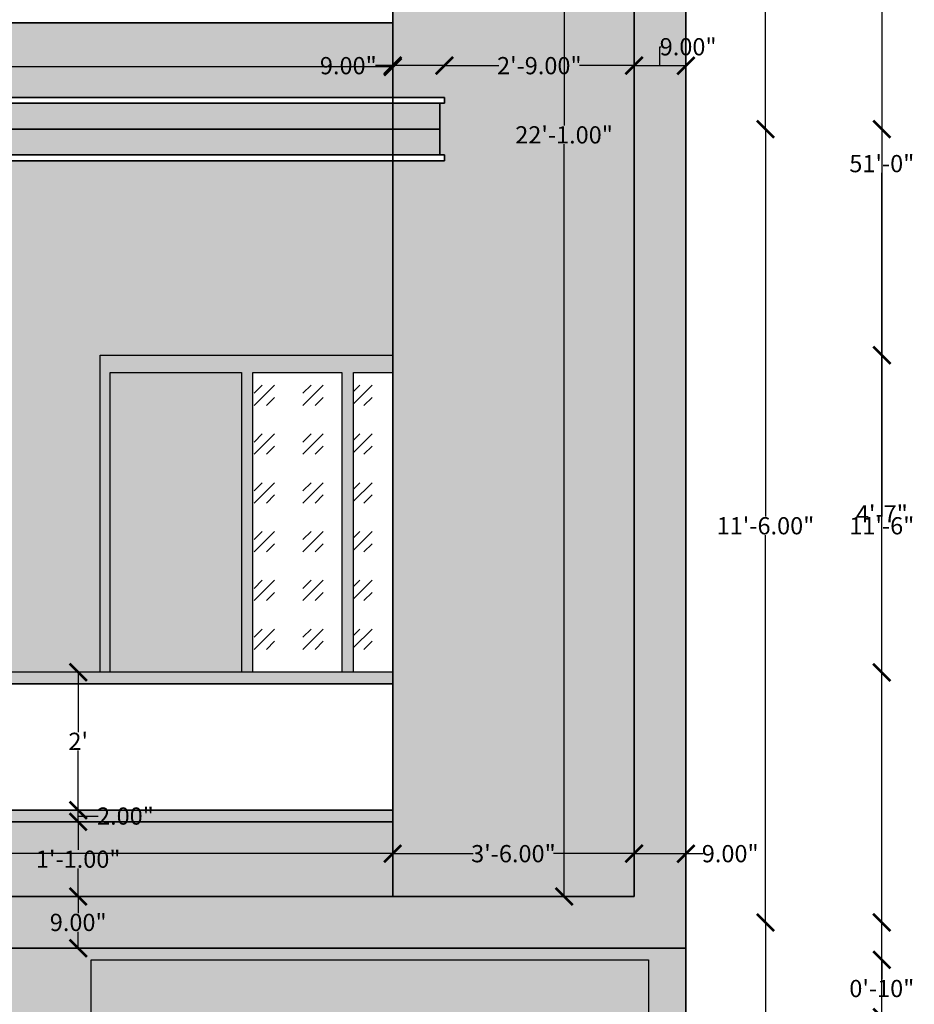
# Model space of a CAD drawing. Units: inches. Extents: x -654 to 390, y -40 to 648.
# Tile 8 of 13: x 231 to 386, y 159 to 330. Entities that reach past the tile are written whole.
import ezdxf

# ---------------------------------------------------------------- set-up
doc = ezdxf.new("R2010")
doc.units = ezdxf.units.IN
doc.header["$PDMODE"] = 3
for name, color, linetype, lineweight in [('A-ANNO-DIMS', 2, 'Continuous', 18), ('A-DOOR', 3, 'Continuous', 25), ('A-ELEV', 7, 'Continuous', 35), ('A-ELEV-FILL', 252, 'Continuous', 13), ('A-ELEV-PATT', 8, 'Continuous', 13), ('A-GLAZ', 4, 'Continuous', 25)]:
    doc.layers.add(name, color=color, linetype=linetype, lineweight=lineweight)
doc.styles.get("Standard").update_dxf_attribs({"font": 'arial.ttf'})
doc.dimstyles.get("Standard").update_dxf_attribs({"dimtxt": 3, "dimasz": 3, "dimexe": 0.18, "dimexo": 0.0625, "dimgap": 0.09, "dimtad": 0, "dimtih": 1, "dimtoh": 1, "dimzin": 0, "dimdsep": 46, "dimlunit": 3, "dimtxsty": 'Standard', "dimblk": 'ARCHTICK', "dimcen": 0.09, "dimse1": 1, "dimse2": 1, "dimadec": 0, "dimazin": 0, "dimtfac": 1, "dimtofl": 0, "dimtmove": 0, "dimatfit": 3, "dimfxl": 1, "dimtolj": 1, "dimtzin": 0, "dimarcsym": 0})

# ---------------------------------------------------------------- blocks, each defined once
blk = doc.blocks.new('_ArchTick')
at = {"color": 0, "linetype": 'ByBlock', "const_width": 0.15}
blk.add_lwpolyline([(-0.5, -0.5), (0.5, 0.5)], dxfattribs=at)
blk = doc.blocks.new('*D4')
at = {"layer": 'A-ANNO-DIMS', "color": 0, "lineweight": -2, "transparency": 16777216}
for p, q in [((360.51, 173.13), (360.51, 105.76)), ((360.51, 35.13), (360.51, 102.51))]:
    blk.add_line(p, q, dxfattribs=at)
at = {"layer": 'Defpoints', "color": 0, "transparency": 16777216}
for p in [(346.65, 173.13), (360.51, 173.13), (346.65, 35.13)]:
    blk.add_point(p, dxfattribs=at)
at = {"layer": 'A-ANNO-DIMS', "color": 0, "lineweight": -2, "transparency": 16777216, "xscale": 3, "yscale": 3, "zscale": 3}
for p, rotation in [((360.51, 173.13), 90), ((360.51, 35.13), 270)]:
    blk.add_blockref('_ArchTick', p, dxfattribs=dict(at, rotation=rotation))
at = {"layer": 'A-ANNO-DIMS', "color": 0, "transparency": 16777216, "insert": (360.51, 104.13), "char_height": 3, "attachment_point": 5}
blk.add_mtext('\\A1;11\'-6.00"', dxfattribs=at)
blk = doc.blocks.new('*D5')
at = {"layer": 'A-ANNO-DIMS', "color": 0, "lineweight": -2, "transparency": 16777216}
for p, q in [((360.51, 311.13), (360.51, 243.76)), ((360.51, 173.13), (360.51, 240.51))]:
    blk.add_line(p, q, dxfattribs=at)
at = {"layer": 'Defpoints', "color": 0, "transparency": 16777216}
for p in [(303.82, 311.13), (360.51, 311.13), (346.65, 173.13)]:
    blk.add_point(p, dxfattribs=at)
at = {"layer": 'A-ANNO-DIMS', "color": 0, "lineweight": -2, "transparency": 16777216, "xscale": 3, "yscale": 3, "zscale": 3}
for p, rotation in [((360.51, 311.13), 90), ((360.51, 173.13), 270)]:
    blk.add_blockref('_ArchTick', p, dxfattribs=dict(at, rotation=rotation))
at = {"layer": 'A-ANNO-DIMS', "color": 0, "transparency": 16777216, "insert": (360.51, 242.13), "char_height": 3, "attachment_point": 5}
blk.add_mtext('\\A1;11\'-6.00"', dxfattribs=at)
blk = doc.blocks.new('*D6')
at = {"layer": 'A-ANNO-DIMS', "color": 0, "lineweight": -2, "transparency": 16777216}
for p, q in [((360.51, 449.13), (360.51, 381.76)), ((360.51, 311.13), (360.51, 378.51))]:
    blk.add_line(p, q, dxfattribs=at)
at = {"layer": 'Defpoints', "color": 0, "transparency": 16777216}
for p in [(337.55, 449.13), (360.51, 449.13), (303.82, 311.13)]:
    blk.add_point(p, dxfattribs=at)
at = {"layer": 'A-ANNO-DIMS', "color": 0, "lineweight": -2, "transparency": 16777216, "xscale": 3, "yscale": 3, "zscale": 3}
for p, rotation in [((360.51, 449.13), 90), ((360.51, 311.13), 270)]:
    blk.add_blockref('_ArchTick', p, dxfattribs=dict(at, rotation=rotation))
at = {"layer": 'A-ANNO-DIMS', "color": 0, "transparency": 16777216, "insert": (360.51, 380.13), "char_height": 3, "attachment_point": 5}
blk.add_mtext('\\A1;11\'-6.00"', dxfattribs=at)
blk = doc.blocks.new('*D41')
at = {"layer": 'A-ANNO-DIMS', "color": 0, "lineweight": -2, "transparency": 16777216}
for p, q in [((325.46, 442.63), (325.46, 311.76)), ((325.46, 177.63), (325.46, 308.51))]:
    blk.add_line(p, q, dxfattribs=at)
at = {"layer": 'Defpoints', "color": 0, "transparency": 16777216}
for p in [(295.65, 442.63), (295.65, 177.63), (325.46, 177.63)]:
    blk.add_point(p, dxfattribs=at)
at = {"layer": 'A-ANNO-DIMS', "color": 0, "lineweight": -2, "transparency": 16777216, "xscale": 3, "yscale": 3, "zscale": 3}
for p, rotation in [((325.46, 442.63), 90), ((325.46, 177.63), 270)]:
    blk.add_blockref('_ArchTick', p, dxfattribs=dict(at, rotation=rotation))
at = {"layer": 'A-ANNO-DIMS', "color": 0, "transparency": 16777216, "insert": (325.46, 310.13), "char_height": 3, "attachment_point": 5}
blk.add_mtext('\\A1;22\'-1.00"', dxfattribs=at)
blk = doc.blocks.new('*D42')
at = {"layer": 'A-ANNO-DIMS', "color": 0, "lineweight": -2, "transparency": 16777216}
for p, q in [((304.65, 322.17), (314.13, 322.17)), ((337.65, 322.17), (328.16, 322.17))]:
    blk.add_line(p, q, dxfattribs=at)
at = {"layer": 'Defpoints', "color": 0, "transparency": 16777216}
for p in [(337.65, 322.17), (304.65, 316.63), (337.65, 316.63)]:
    blk.add_point(p, dxfattribs=at)
at = {"layer": 'A-ANNO-DIMS', "color": 0, "lineweight": -2, "transparency": 16777216, "xscale": 3, "yscale": 3, "zscale": 3, "rotation": 180}
blk.add_blockref('_ArchTick', (304.65, 322.17), dxfattribs=at)
at = {"layer": 'A-ANNO-DIMS', "color": 0, "lineweight": -2, "transparency": 16777216, "xscale": 3, "yscale": 3, "zscale": 3}
blk.add_blockref('_ArchTick', (337.65, 322.17), dxfattribs=at)
at = {"layer": 'A-ANNO-DIMS', "color": 0, "transparency": 16777216, "insert": (321.15, 322.17), "char_height": 3, "attachment_point": 5}
blk.add_mtext('\\A1;2\'-9.00"', dxfattribs=at)
blk = doc.blocks.new('*D43')
at = {"layer": 'A-ANNO-DIMS', "color": 0, "lineweight": -2, "transparency": 16777216}
for p, q in [((342.15, 322.17), (342.15, 325.46)), ((342.15, 325.46), (342.33, 325.46)), ((337.65, 322.17), (346.65, 322.17))]:
    blk.add_line(p, q, dxfattribs=at)
at = {"layer": 'Defpoints', "color": 0, "transparency": 16777216}
for p in [(346.65, 322.17), (346.65, 322.17), (337.65, 316.63)]:
    blk.add_point(p, dxfattribs=at)
at = {"layer": 'A-ANNO-DIMS', "color": 0, "lineweight": -2, "transparency": 16777216, "xscale": 3, "yscale": 3, "zscale": 3, "rotation": 180}
blk.add_blockref('_ArchTick', (337.65, 322.17), dxfattribs=at)
at = {"layer": 'A-ANNO-DIMS', "color": 0, "lineweight": -2, "transparency": 16777216, "xscale": 3, "yscale": 3, "zscale": 3}
blk.add_blockref('_ArchTick', (346.65, 322.17), dxfattribs=at)
at = {"layer": 'A-ANNO-DIMS', "color": 0, "transparency": 16777216, "insert": (347.05, 325.46), "char_height": 3, "attachment_point": 5}
blk.add_mtext('\\A1;9.00"', dxfattribs=at)
blk = doc.blocks.new('*D44')
at = {"layer": 'A-ANNO-DIMS', "color": 0, "lineweight": -2, "transparency": 16777216}
for p, q in [((295.65, 322.17), (292.65, 322.17)), ((304.65, 322.17), (295.65, 322.17))]:
    blk.add_line(p, q, dxfattribs=at)
at = {"layer": 'Defpoints', "color": 0, "transparency": 16777216}
for p in [(295.65, 322.17), (295.65, 316.63), (304.65, 316.63)]:
    blk.add_point(p, dxfattribs=at)
at = {"layer": 'A-ANNO-DIMS', "color": 0, "lineweight": -2, "transparency": 16777216, "xscale": 3, "yscale": 3, "zscale": 3, "rotation": 180}
blk.add_blockref('_ArchTick', (295.65, 322.17), dxfattribs=at)
at = {"layer": 'A-ANNO-DIMS', "color": 0, "lineweight": -2, "transparency": 16777216, "xscale": 3, "yscale": 3, "zscale": 3}
blk.add_blockref('_ArchTick', (304.65, 322.17), dxfattribs=at)
at = {"layer": 'A-ANNO-DIMS', "color": 0, "transparency": 16777216, "insert": (287.92, 322.17), "char_height": 3, "attachment_point": 5}
blk.add_mtext('\\A1;9.00"', dxfattribs=at)
blk = doc.blocks.new('*D46')
at = {"layer": 'A-ANNO-DIMS', "color": 0, "lineweight": -2, "transparency": 16777216}
for p, q in [((145.65, 321.96), (212.63, 321.96)), ((295.65, 321.96), (228.66, 321.96))]:
    blk.add_line(p, q, dxfattribs=at)
at = {"layer": 'Defpoints', "color": 0, "transparency": 16777216}
for p in [(145.65, 329.63), (145.65, 321.96), (295.65, 316.63)]:
    blk.add_point(p, dxfattribs=at)
at = {"layer": 'A-ANNO-DIMS', "color": 0, "lineweight": -2, "transparency": 16777216, "xscale": 3, "yscale": 3, "zscale": 3, "rotation": 180}
blk.add_blockref('_ArchTick', (145.65, 321.96), dxfattribs=at)
at = {"layer": 'A-ANNO-DIMS', "color": 0, "lineweight": -2, "transparency": 16777216, "xscale": 3, "yscale": 3, "zscale": 3}
blk.add_blockref('_ArchTick', (295.65, 321.96), dxfattribs=at)
at = {"layer": 'A-ANNO-DIMS', "color": 0, "transparency": 16777216, "insert": (220.65, 321.96), "char_height": 3, "attachment_point": 5}
blk.add_mtext('\\A1;12\'-6.00"', dxfattribs=at)
blk = doc.blocks.new('*D58')
at = {"layer": 'A-ANNO-DIMS', "color": 0, "lineweight": -2, "transparency": 16777216}
for p, q in [((337.65, 185.09), (346.65, 185.09)), ((346.65, 185.09), (349.65, 185.09))]:
    blk.add_line(p, q, dxfattribs=at)
at = {"layer": 'Defpoints', "color": 0, "transparency": 16777216}
for p in [(346.65, 185.09), (337.65, 177.63), (346.65, 177.63)]:
    blk.add_point(p, dxfattribs=at)
at = {"layer": 'A-ANNO-DIMS', "color": 0, "lineweight": -2, "transparency": 16777216, "xscale": 3, "yscale": 3, "zscale": 3, "rotation": 180}
blk.add_blockref('_ArchTick', (337.65, 185.09), dxfattribs=at)
at = {"layer": 'A-ANNO-DIMS', "color": 0, "lineweight": -2, "transparency": 16777216, "xscale": 3, "yscale": 3, "zscale": 3}
blk.add_blockref('_ArchTick', (346.65, 185.09), dxfattribs=at)
at = {"layer": 'A-ANNO-DIMS', "color": 0, "transparency": 16777216, "insert": (354.37, 185.09), "char_height": 3, "attachment_point": 5}
blk.add_mtext('\\A1;9.00"', dxfattribs=at)
blk = doc.blocks.new('*D59')
at = {"layer": 'A-ANNO-DIMS', "color": 0, "lineweight": -2, "transparency": 16777216}
for p, q in [((295.65, 185.09), (309.66, 185.09)), ((337.65, 185.09), (323.64, 185.09))]:
    blk.add_line(p, q, dxfattribs=at)
at = {"layer": 'Defpoints', "color": 0, "transparency": 16777216}
for p in [(295.65, 185.09), (295.65, 185.09), (337.65, 185.09)]:
    blk.add_point(p, dxfattribs=at)
at = {"layer": 'A-ANNO-DIMS', "color": 0, "lineweight": -2, "transparency": 16777216, "xscale": 3, "yscale": 3, "zscale": 3, "rotation": 180}
blk.add_blockref('_ArchTick', (295.65, 185.09), dxfattribs=at)
at = {"layer": 'A-ANNO-DIMS', "color": 0, "lineweight": -2, "transparency": 16777216, "xscale": 3, "yscale": 3, "zscale": 3}
blk.add_blockref('_ArchTick', (337.65, 185.09), dxfattribs=at)
at = {"layer": 'A-ANNO-DIMS', "color": 0, "transparency": 16777216, "insert": (316.65, 185.09), "char_height": 3, "attachment_point": 5}
blk.add_mtext('\\A1;3\'-6.00"', dxfattribs=at)
blk = doc.blocks.new('*D60')
at = {"layer": 'A-ANNO-DIMS', "color": 0, "lineweight": -2, "transparency": 16777216}
for p, q in [((120.15, 185.09), (199.88, 185.09)), ((295.65, 185.09), (215.91, 185.09))]:
    blk.add_line(p, q, dxfattribs=at)
at = {"layer": 'Defpoints', "color": 0, "transparency": 16777216}
for p in [(120.15, 185.09), (120.15, 185.09), (295.65, 185.09)]:
    blk.add_point(p, dxfattribs=at)
at = {"layer": 'A-ANNO-DIMS', "color": 0, "lineweight": -2, "transparency": 16777216, "xscale": 3, "yscale": 3, "zscale": 3, "rotation": 180}
blk.add_blockref('_ArchTick', (120.15, 185.09), dxfattribs=at)
at = {"layer": 'A-ANNO-DIMS', "color": 0, "lineweight": -2, "transparency": 16777216, "xscale": 3, "yscale": 3, "zscale": 3}
blk.add_blockref('_ArchTick', (295.65, 185.09), dxfattribs=at)
at = {"layer": 'A-ANNO-DIMS', "color": 0, "transparency": 16777216, "insert": (207.9, 185.09), "char_height": 3, "attachment_point": 5}
blk.add_mtext('\\A1;14\'-7.50"', dxfattribs=at)
blk = doc.blocks.new('*D62')
at = {"layer": 'A-ANNO-DIMS', "color": 0, "lineweight": -2, "transparency": 16777216}
for p, q in [((240.92, 190.63), (240.92, 185.76)), ((240.92, 177.63), (240.92, 182.51))]:
    blk.add_line(p, q, dxfattribs=at)
at = {"layer": 'Defpoints', "color": 0, "transparency": 16777216}
for p in [(240.92, 190.63), (295.65, 190.63), (295.65, 177.63)]:
    blk.add_point(p, dxfattribs=at)
at = {"layer": 'A-ANNO-DIMS', "color": 0, "lineweight": -2, "transparency": 16777216, "xscale": 3, "yscale": 3, "zscale": 3}
for p, rotation in [((240.92, 190.63), 90), ((240.92, 177.63), 270)]:
    blk.add_blockref('_ArchTick', p, dxfattribs=dict(at, rotation=rotation))
at = {"layer": 'A-ANNO-DIMS', "color": 0, "transparency": 16777216, "insert": (240.92, 184.13), "char_height": 3, "attachment_point": 5}
blk.add_mtext('\\A1;1\'-1.00"', dxfattribs=at)
blk = doc.blocks.new('*D63')
at = {"layer": 'A-ANNO-DIMS', "color": 0, "lineweight": -2, "transparency": 16777216}
for p, q in [((240.92, 190.63), (240.92, 192.63)), ((240.92, 191.63), (244.21, 191.63)), ((244.21, 191.63), (244.39, 191.63))]:
    blk.add_line(p, q, dxfattribs=at)
at = {"layer": 'Defpoints', "color": 0, "transparency": 16777216}
for p in [(240.92, 192.63), (240.92, 192.63), (295.65, 190.63)]:
    blk.add_point(p, dxfattribs=at)
at = {"layer": 'A-ANNO-DIMS', "color": 0, "lineweight": -2, "transparency": 16777216, "xscale": 3, "yscale": 3, "zscale": 3}
for p, rotation in [((240.92, 192.63), 90), ((240.92, 190.63), 270)]:
    blk.add_blockref('_ArchTick', p, dxfattribs=dict(at, rotation=rotation))
at = {"layer": 'A-ANNO-DIMS', "color": 0, "transparency": 16777216, "insert": (249.14, 191.63), "char_height": 3, "attachment_point": 5}
blk.add_mtext('\\A1;2.00"', dxfattribs=at)
blk = doc.blocks.new('*D64')
at = {"layer": 'A-ANNO-DIMS', "color": 0, "lineweight": -2, "transparency": 16777216}
for p, q in [((240.92, 216.63), (240.92, 206.23)), ((240.92, 192.63), (240.92, 203.04))]:
    blk.add_line(p, q, dxfattribs=at)
at = {"layer": 'Defpoints', "color": 0, "transparency": 16777216}
for p in [(240.92, 216.63), (240.92, 216.63), (240.92, 192.63)]:
    blk.add_point(p, dxfattribs=at)
at = {"layer": 'A-ANNO-DIMS', "color": 0, "lineweight": -2, "transparency": 16777216, "xscale": 3, "yscale": 3, "zscale": 3}
for p, rotation in [((240.92, 216.63), 90), ((240.92, 192.63), 270)]:
    blk.add_blockref('_ArchTick', p, dxfattribs=dict(at, rotation=rotation))
at = {"layer": 'A-ANNO-DIMS', "color": 0, "transparency": 16777216, "insert": (240.92, 204.63), "char_height": 3, "attachment_point": 5}
blk.add_mtext("\\A1;2'", dxfattribs=at)
blk = doc.blocks.new('*D71')
at = {"layer": 'A-ANNO-DIMS', "color": 0, "lineweight": -2, "transparency": 16777216}
for p, q in [((240.92, 177.63), (240.92, 174.76)), ((240.92, 168.63), (240.92, 171.51))]:
    blk.add_line(p, q, dxfattribs=at)
at = {"layer": 'Defpoints', "color": 0, "transparency": 16777216}
for p in [(240.92, 177.63), (240.92, 168.63), (240.92, 168.63)]:
    blk.add_point(p, dxfattribs=at)
at = {"layer": 'A-ANNO-DIMS', "color": 0, "lineweight": -2, "transparency": 16777216, "xscale": 3, "yscale": 3, "zscale": 3}
for p, rotation in [((240.92, 177.63), 90), ((240.92, 168.63), 270)]:
    blk.add_blockref('_ArchTick', p, dxfattribs=dict(at, rotation=rotation))
at = {"layer": 'A-ANNO-DIMS', "color": 0, "transparency": 16777216, "insert": (240.92, 173.13), "char_height": 3, "attachment_point": 5}
blk.add_mtext('\\A1;9.00"', dxfattribs=at)
blk = doc.blocks.new('*D76')
at = {"layer": 'A-ANNO-DIMS', "color": 0, "lineweight": -2, "transparency": 16777216}
for p, q in [((380.75, 611.13), (380.75, 306.76)), ((380.75, -0.87), (380.75, 303.51))]:
    blk.add_line(p, q, dxfattribs=at)
at = {"layer": 'Defpoints', "color": 0, "transparency": 16777216}
for p in [(126.65, 611.13), (380.75, 611.13), (346.65, -0.87)]:
    blk.add_point(p, dxfattribs=at)
at = {"layer": 'A-ANNO-DIMS', "color": 0, "lineweight": -2, "transparency": 16777216, "xscale": 3, "yscale": 3, "zscale": 3}
for p, rotation in [((380.75, 611.13), 90), ((380.75, -0.87), 270)]:
    blk.add_blockref('_ArchTick', p, dxfattribs=dict(at, rotation=rotation))
at = {"layer": 'A-ANNO-DIMS', "color": 0, "transparency": 16777216, "insert": (380.75, 305.13), "char_height": 3, "attachment_point": 5}
blk.add_mtext('\\A1;51\'-0"', dxfattribs=at)
blk = doc.blocks.new('*D89')
at = {"layer": 'A-ANNO-DIMS', "color": 0, "lineweight": -2, "transparency": 16777216}
for p, q in [((243.65, 643.23), (287.57, 643.23)), ((339.65, 643.23), (295.73, 643.23))]:
    blk.add_line(p, q, dxfattribs=at)
at = {"layer": 'Defpoints', "color": 0, "transparency": 16777216}
for p in [(339.65, 643.23), (243.65, 17.13), (339.65, 17.13)]:
    blk.add_point(p, dxfattribs=at)
at = {"layer": 'A-ANNO-DIMS', "color": 0, "lineweight": -2, "transparency": 16777216, "xscale": 3, "yscale": 3, "zscale": 3, "rotation": 180}
blk.add_blockref('_ArchTick', (243.65, 643.23), dxfattribs=at)
at = {"layer": 'A-ANNO-DIMS', "color": 0, "lineweight": -2, "transparency": 16777216, "xscale": 3, "yscale": 3, "zscale": 3}
blk.add_blockref('_ArchTick', (339.65, 643.23), dxfattribs=at)
at = {"layer": 'A-ANNO-DIMS', "color": 0, "transparency": 16777216, "insert": (291.65, 643.23), "char_height": 3, "attachment_point": 5}
blk.add_mtext('\\A1;8\'-0"', dxfattribs=at)
blk = doc.blocks.new('*D90')
at = {"layer": 'A-ANNO-DIMS', "color": 0, "lineweight": -2, "transparency": 16777216}
for p, q in [((339.65, 643.23), (346.65, 643.23)), ((346.65, 643.23), (349.65, 643.23))]:
    blk.add_line(p, q, dxfattribs=at)
at = {"layer": 'Defpoints', "color": 0, "transparency": 16777216}
for p in [(346.65, 643.23), (339.65, 17.13), (346.65, 17.13)]:
    blk.add_point(p, dxfattribs=at)
at = {"layer": 'A-ANNO-DIMS', "color": 0, "lineweight": -2, "transparency": 16777216, "xscale": 3, "yscale": 3, "zscale": 3, "rotation": 180}
blk.add_blockref('_ArchTick', (339.65, 643.23), dxfattribs=at)
at = {"layer": 'A-ANNO-DIMS', "color": 0, "lineweight": -2, "transparency": 16777216, "xscale": 3, "yscale": 3, "zscale": 3}
blk.add_blockref('_ArchTick', (346.65, 643.23), dxfattribs=at)
at = {"layer": 'A-ANNO-DIMS', "color": 0, "transparency": 16777216, "insert": (353.72, 643.23), "char_height": 3, "attachment_point": 5}
blk.add_mtext('\\A1;0\'-7"', dxfattribs=at)
blk = doc.blocks.new('*D91')
at = {"layer": 'A-ANNO-DIMS', "color": 0, "lineweight": -2, "transparency": 16777216}
for p, q in [((380.75, 166.63), (380.75, 163.26)), ((380.75, 156.63), (380.75, 160.01))]:
    blk.add_line(p, q, dxfattribs=at)
at = {"layer": 'Defpoints', "color": 0, "transparency": 16777216}
for p in [(243.15, 166.63), (380.75, 166.63), (243.15, 156.63)]:
    blk.add_point(p, dxfattribs=at)
at = {"layer": 'A-ANNO-DIMS', "color": 0, "lineweight": -2, "transparency": 16777216, "xscale": 3, "yscale": 3, "zscale": 3}
for p, rotation in [((380.75, 166.63), 90), ((380.75, 156.63), 270)]:
    blk.add_blockref('_ArchTick', p, dxfattribs=dict(at, rotation=rotation))
at = {"layer": 'A-ANNO-DIMS', "color": 0, "transparency": 16777216, "insert": (380.75, 161.63), "char_height": 3, "attachment_point": 5}
blk.add_mtext('\\A1;0\'-10"', dxfattribs=at)
blk = doc.blocks.new('*D94')
at = {"layer": 'A-ANNO-DIMS', "color": 0, "lineweight": -2, "transparency": 16777216}
for p, q in [((380.75, 271.79), (380.75, 245.8)), ((380.75, 216.63), (380.75, 242.62))]:
    blk.add_line(p, q, dxfattribs=at)
at = {"layer": 'Defpoints', "color": 0, "transparency": 16777216}
for p in [(221.33, 271.79), (244.73, 216.63), (380.75, 216.63)]:
    blk.add_point(p, dxfattribs=at)
at = {"layer": 'A-ANNO-DIMS', "color": 0, "lineweight": -2, "transparency": 16777216, "xscale": 3, "yscale": 3, "zscale": 3}
for p, rotation in [((380.75, 271.79), 90), ((380.75, 216.63), 270)]:
    blk.add_blockref('_ArchTick', p, dxfattribs=dict(at, rotation=rotation))
at = {"layer": 'A-ANNO-DIMS', "color": 0, "transparency": 16777216, "insert": (380.75, 244.21), "char_height": 3, "attachment_point": 5}
blk.add_mtext('\\A1;4\'-7"', dxfattribs=at)
blk = doc.blocks.new('*D95')
at = {"layer": 'A-ANNO-DIMS', "color": 0, "lineweight": -2, "transparency": 16777216}
for p, q in [((244.73, -32.97), (266.05, -32.97)), ((295.65, -32.97), (274.32, -32.97))]:
    blk.add_line(p, q, dxfattribs=at)
at = {"layer": 'Defpoints', "color": 0, "transparency": 16777216}
for p in [(244.73, 271.79), (295.65, 271.79), (295.65, -32.97)]:
    blk.add_point(p, dxfattribs=at)
at = {"layer": 'A-ANNO-DIMS', "color": 0, "lineweight": -2, "transparency": 16777216, "xscale": 3, "yscale": 3, "zscale": 3, "rotation": 180}
blk.add_blockref('_ArchTick', (244.73, -32.97), dxfattribs=at)
at = {"layer": 'A-ANNO-DIMS', "color": 0, "lineweight": -2, "transparency": 16777216, "xscale": 3, "yscale": 3, "zscale": 3}
blk.add_blockref('_ArchTick', (295.65, -32.97), dxfattribs=at)
at = {"layer": 'A-ANNO-DIMS', "color": 0, "transparency": 16777216, "insert": (270.19, -32.97), "char_height": 3, "attachment_point": 5}
blk.add_mtext('\\A1;4\'-3"', dxfattribs=at)
blk = doc.blocks.new('*D99')
at = {"layer": 'A-ANNO-DIMS', "color": 0, "lineweight": -2, "transparency": 16777216}
for p, q in [((380.75, 311.13), (380.75, 243.76)), ((380.75, 173.13), (380.75, 240.51))]:
    blk.add_line(p, q, dxfattribs=at)
at = {"layer": 'Defpoints', "color": 0, "transparency": 16777216}
for p in [(178.74, 311.13), (380.75, 311.13), (178.74, 173.13)]:
    blk.add_point(p, dxfattribs=at)
at = {"layer": 'A-ANNO-DIMS', "color": 0, "lineweight": -2, "transparency": 16777216, "xscale": 3, "yscale": 3, "zscale": 3}
for p, rotation in [((380.75, 311.13), 90), ((380.75, 173.13), 270)]:
    blk.add_blockref('_ArchTick', p, dxfattribs=dict(at, rotation=rotation))
at = {"layer": 'A-ANNO-DIMS', "color": 0, "transparency": 16777216, "insert": (380.75, 242.13), "char_height": 3, "attachment_point": 5}
blk.add_mtext('\\A1;11\'-6"', dxfattribs=at)
blk = doc.blocks.new('*D102')
at = {"layer": 'A-ANNO-DIMS', "color": 0, "lineweight": -2, "transparency": 16777216}
for p, q in [((179.88, -32.97), (205.8, -32.97)), ((239.87, -32.97), (213.95, -32.97))]:
    blk.add_line(p, q, dxfattribs=at)
at = {"layer": 'Defpoints', "color": 0, "transparency": 16777216}
for p in [(179.88, 355.63), (239.87, 355.63), (239.87, -32.97)]:
    blk.add_point(p, dxfattribs=at)
at = {"layer": 'A-ANNO-DIMS', "color": 0, "lineweight": -2, "transparency": 16777216, "xscale": 3, "yscale": 3, "zscale": 3, "rotation": 180}
blk.add_blockref('_ArchTick', (179.88, -32.97), dxfattribs=at)
at = {"layer": 'A-ANNO-DIMS', "color": 0, "lineweight": -2, "transparency": 16777216, "xscale": 3, "yscale": 3, "zscale": 3}
blk.add_blockref('_ArchTick', (239.87, -32.97), dxfattribs=at)
at = {"layer": 'A-ANNO-DIMS', "color": 0, "transparency": 16777216, "insert": (209.87, -32.97), "char_height": 3, "attachment_point": 5}
blk.add_mtext('\\A1;5\'-0"', dxfattribs=at)
blk = doc.blocks.new('*D103')
at = {"layer": 'A-ANNO-DIMS', "color": 0, "lineweight": -2, "transparency": 16777216}
for p, q in [((239.87, -32.97), (257.87, -32.97)), ((291.14, -32.97), (273.14, -32.97))]:
    blk.add_line(p, q, dxfattribs=at)
at = {"layer": 'Defpoints', "color": 0, "transparency": 16777216}
for p in [(239.87, 355.63), (291.14, 355.63), (291.14, -32.97)]:
    blk.add_point(p, dxfattribs=at)
at = {"layer": 'A-ANNO-DIMS', "color": 0, "lineweight": -2, "transparency": 16777216, "xscale": 3, "yscale": 3, "zscale": 3, "rotation": 180}
blk.add_blockref('_ArchTick', (239.87, -32.97), dxfattribs=at)
at = {"layer": 'A-ANNO-DIMS', "color": 0, "lineweight": -2, "transparency": 16777216, "xscale": 3, "yscale": 3, "zscale": 3}
blk.add_blockref('_ArchTick', (291.14, -32.97), dxfattribs=at)
at = {"layer": 'A-ANNO-DIMS', "color": 0, "transparency": 16777216, "insert": (265.51, -32.97), "char_height": 3, "attachment_point": 5}
blk.add_mtext('\\A1;4\'-3 1/2"', dxfattribs=at)

msp = doc.modelspace()

# ---------------------------------------------------------------- hatches: boundary and pattern name
at = {"layer": 'A-ELEV-FILL'}
h = msp.add_hatch(color=256, dxfattribs=at)
h.dxf.hatch_style = 1
h.paths.add_polyline_path([(161.035, 590.134), (-1.354, 590.134), (-1.354, 581.134), (161.035, 581.134)])
h.paths.add_polyline_path([(346.646, 453.634), (-1.354, 453.634), (-1.354, 444.634), (337.646, 444.634), (337.646, 177.634), (178.742, 177.634), (178.742, 173.134), (176.742, 173.134), (176.742, 177.634), (166.742, 177.634), (166.742, 173.134), (164.742, 173.134), (164.742, 177.634), (154.742, 177.634), (154.742, 173.134), (152.742, 173.134), (152.742, 177.634), (142.742, 177.634), (142.742, 173.134), (140.742, 173.134), (140.742, 177.634), (130.742, 177.634), (130.742, 173.134), (128.742, 173.134), (128.742, 177.634), (115.646, 177.634), (115.646, 168.634), (346.646, 168.634), (346.646, 173.134)])
h.paths.add_polyline_path([(7.646, 87.642), (-1.354, 87.642), (-1.354, 17.134), (7.646, 17.134)])
h.paths.add_polyline_path([(16.396, 116.134), (60.646, 116.134), (60.646, 83.134), (62.646, 83.134), (113.646, 83.134), (115.646, 83.134), (115.646, 125.134), (7.646, 125.134), (7.646, 89.642), (8.146, 89.642), (8.146, 87.642), (7.646, 87.642), (7.646, 83.134), (9.646, 83.134), (16.396, 83.134)])
h = msp.add_hatch(color=256, dxfattribs=at)
h.dxf.hatch_style = 1
h.paths.add_polyline_path([(346.646, 587.634), (161.035, 587.634), (161.035, 583.634), (342.646, 583.634), (342.646, 497.134), (346.646, 497.134), (346.646, 583.634)])
h.paths.add_polyline_path([(295.646, 315.634), (98.293, 315.634), (98.293, 311.134), (295.646, 311.134)])
h.paths.add_polyline_path([(128.742, 311.134), (98.293, 311.134), (98.293, 306.634), (128.742, 306.634)])
h.paths.add_polyline_path([(140.742, 311.134), (130.742, 311.134), (130.742, 306.634), (140.742, 306.634)])
h.paths.add_polyline_path([(152.742, 311.134), (142.742, 311.134), (142.742, 306.634), (152.742, 306.634)])
h.paths.add_polyline_path([(164.742, 311.134), (154.742, 311.134), (154.742, 306.634), (164.742, 306.634)])
h.paths.add_polyline_path([(176.742, 311.134), (166.742, 311.134), (166.742, 306.634), (176.742, 306.634)])
h.paths.add_polyline_path([(295.646, 311.134), (178.742, 311.134), (178.742, 306.634), (295.646, 306.634)])
h.paths.add_polyline_path([(303.818, 315.634), (295.646, 315.634), (295.646, 311.134), (303.818, 311.134)])
h.paths.add_polyline_path([(303.818, 311.134), (295.646, 311.134), (295.646, 306.634), (303.818, 306.634)])
h = msp.add_hatch(color=256, dxfattribs=at)
h.dxf.hatch_style = 1
h.paths.add_polyline_path([(41.55, 80.08), (28.05, 80.08), (28.05, 20.08), (41.55, 20.08)])
h.paths.add_polyline_path([(93.843, 80.08), (80.343, 80.08), (80.343, 20.08), (93.843, 20.08)])
h.paths.add_polyline_path([(337.646, 442.634), (295.646, 442.634), (295.646, 316.634), (304.646, 316.634), (304.646, 315.634), (303.818, 315.634), (303.818, 306.634), (304.646, 306.634), (304.646, 305.634), (295.646, 305.634), (295.646, 177.634), (337.646, 177.634)])
h.paths.add_polyline_path([(346.646, 495.134), (184.646, 495.134), (184.646, 453.634), (346.646, 453.634)])
h.paths.add_polyline_path([(198.646, 473.634), (198.646, 486.134), (332.646, 486.134), (332.646, 473.634)], flags=16)
h.paths.add_polyline_path([(199.646, 474.634), (199.646, 485.134), (331.646, 485.134), (331.646, 474.634)], flags=0)
h = msp.add_hatch(color=256, dxfattribs=at)
h.dxf.hatch_style = 1
h.paths.add_polyline_path([(295.646, 190.634), (178.742, 190.634), (178.742, 177.634), (295.646, 177.634)])
h.paths.add_polyline_path([(176.742, 190.634), (166.742, 190.634), (166.742, 177.634), (176.742, 177.634)])
h.paths.add_polyline_path([(164.742, 190.634), (154.742, 190.634), (154.742, 177.634), (164.742, 177.634)])
h.paths.add_polyline_path([(152.742, 190.634), (142.742, 190.634), (142.742, 177.634), (152.742, 177.634)])
h.paths.add_polyline_path([(140.742, 190.634), (130.742, 190.634), (130.742, 177.634), (140.742, 177.634)])
h.paths.add_polyline_path([(128.742, 190.634), (120.146, 190.634), (120.146, 177.634), (128.742, 177.634)])
h.paths.add_polyline_path([(295.646, 329.634), (145.646, 329.634), (145.646, 442.634), (100.646, 442.634), (100.646, 316.634), (295.646, 316.634)])
h.paths.add_polyline_path([(138.646, 359.634), (107.646, 359.634), (107.646, 438.634), (138.646, 438.634)], flags=16)
h.paths.add_polyline_path([(136.646, 361.634), (109.646, 361.634), (109.646, 436.634), (136.646, 436.634)], flags=0)
h.paths.add_polyline_path([(184.646, 466.634), (7.646, 466.634), (7.646, 453.634), (184.646, 453.634)])
h.paths.add_polyline_path([(184.646, 494.634), (7.646, 494.634), (7.646, 492.634), (184.646, 492.634)])
h.paths.add_polyline_path([(10.336, 492.634), (9.336, 492.634), (9.336, 468.634), (10.336, 468.634)])
h.paths.add_polyline_path([(17.352, 492.634), (16.352, 492.634), (16.352, 468.634), (17.352, 468.634)])
h.paths.add_polyline_path([(24.368, 492.634), (23.368, 492.634), (23.368, 468.634), (24.368, 468.634)])
h.paths.add_polyline_path([(31.384, 492.634), (30.384, 492.634), (30.384, 468.634), (31.384, 468.634)])
h.paths.add_polyline_path([(38.4, 492.634), (37.4, 492.634), (37.4, 468.634), (38.4, 468.634)])
h.paths.add_polyline_path([(45.416, 492.634), (44.416, 492.634), (44.416, 468.634), (45.416, 468.634)])
h.paths.add_polyline_path([(52.432, 492.634), (51.432, 492.634), (51.432, 468.634), (52.432, 468.634)])
h.paths.add_polyline_path([(59.448, 492.634), (58.448, 492.634), (58.448, 468.634), (59.448, 468.634)])
h.paths.add_polyline_path([(66.464, 492.634), (65.464, 492.634), (65.464, 468.634), (66.464, 468.634)])
h.paths.add_polyline_path([(73.48, 492.634), (72.48, 492.634), (72.48, 468.634), (73.48, 468.634)])
h.paths.add_polyline_path([(80.496, 492.634), (79.496, 492.634), (79.496, 468.634), (80.496, 468.634)])
h.paths.add_polyline_path([(87.512, 492.634), (86.512, 492.634), (86.512, 468.634), (87.512, 468.634)])
h.paths.add_polyline_path([(94.528, 492.634), (93.528, 492.634), (93.528, 468.634), (94.528, 468.634)])
h.paths.add_polyline_path([(101.544, 492.634), (100.544, 492.634), (100.544, 468.634), (101.544, 468.634)])
h.paths.add_polyline_path([(108.559, 492.634), (107.559, 492.634), (107.559, 468.634), (108.559, 468.634)])
h.paths.add_polyline_path([(115.575, 492.634), (114.575, 492.634), (114.575, 468.634), (115.575, 468.634)])
h.paths.add_polyline_path([(122.591, 492.634), (121.591, 492.634), (121.591, 468.634), (122.591, 468.634)])
h.paths.add_polyline_path([(129.607, 492.634), (128.607, 492.634), (128.607, 468.634), (129.607, 468.634)])
h.paths.add_polyline_path([(136.623, 492.634), (135.623, 492.634), (135.623, 468.634), (136.623, 468.634)])
h.paths.add_polyline_path([(143.639, 492.634), (142.639, 492.634), (142.639, 468.634), (143.639, 468.634)])
h.paths.add_polyline_path([(150.655, 492.634), (149.655, 492.634), (149.655, 468.634), (150.655, 468.634)])
h.paths.add_polyline_path([(157.671, 492.634), (156.671, 492.634), (156.671, 468.634), (157.671, 468.634)])
h.paths.add_polyline_path([(164.687, 492.634), (163.687, 492.634), (163.687, 468.634), (164.687, 468.634)])
h.paths.add_polyline_path([(171.703, 492.634), (170.703, 492.634), (170.703, 468.634), (171.703, 468.634)])
h.paths.add_polyline_path([(178.719, 492.634), (177.719, 492.634), (177.719, 468.634), (178.719, 468.634)])
h = msp.add_hatch(color=256, dxfattribs=at)
h.dxf.hatch_style = 1
h.paths.add_polyline_path([(138.646, 438.634), (107.646, 438.634), (107.646, 359.634), (138.646, 359.634)])
h.paths.add_polyline_path([(136.646, 436.634), (136.646, 361.634), (109.646, 361.634), (109.646, 436.634)], flags=16)
h.paths.add_polyline_path([(179.877, 410.786), (145.646, 410.786), (145.646, 407.786), (153.285, 407.786), (153.285, 357.634), (145.646, 357.634), (145.646, 355.634), (179.877, 355.634)])
h.paths.add_polyline_path([(178.123, 407.786), (178.123, 357.634), (155.286, 357.634), (155.286, 407.786)], flags=16)
h.paths.add_polyline_path([(291.141, 410.786), (239.871, 410.786), (239.871, 355.634), (241.996, 355.634), (241.996, 407.786), (269.317, 407.786), (269.317, 355.634), (271.318, 355.634), (271.318, 407.786), (289.369, 407.786), (289.369, 355.634), (291.141, 355.634)])
h.paths.add_polyline_path([(128.225, 268.786), (128.742, 268.786), (128.742, 271.786), (125.225, 271.786), (125.225, 216.634), (128.225, 216.634)])
h.paths.add_polyline_path([(140.742, 271.786), (130.742, 271.786), (130.742, 268.786), (140.742, 268.786)])
h.paths.add_polyline_path([(152.742, 271.786), (142.742, 271.786), (142.742, 268.786), (152.742, 268.786)])
h.paths.add_polyline_path([(164.742, 271.786), (154.742, 271.786), (154.742, 268.786), (164.742, 268.786)])
h.paths.add_polyline_path([(176.742, 271.786), (167.328, 271.786), (166.742, 271.786), (166.742, 268.786), (167.328, 268.786), (167.328, 216.634), (169.328, 216.634), (169.328, 268.786), (176.742, 268.786)])
h.paths.add_polyline_path([(221.328, 271.786), (178.742, 271.786), (178.742, 268.786), (184.828, 268.786), (184.828, 216.634), (186.829, 216.634), (186.829, 268.786), (202.329, 268.786), (202.329, 216.634), (204.325, 216.634), (204.325, 268.786), (219.825, 268.786), (219.825, 216.634), (221.328, 216.634)])
h.paths.add_polyline_path([(295.646, 271.786), (244.726, 271.786), (244.726, 216.634), (246.481, 216.634), (246.481, 268.786), (269.317, 268.786), (269.317, 216.634), (271.318, 216.634), (271.318, 268.786), (286.818, 268.786), (286.818, 216.634), (288.814, 216.634), (288.814, 268.786), (295.646, 268.786)])
h.paths.add_polyline_path([(295.646, 216.634), (178.742, 216.634), (178.742, 214.634), (295.646, 214.634)])
h.paths.add_polyline_path([(128.742, 216.634), (123.485, 216.634), (123.485, 214.634), (128.742, 214.634)])
h.paths.add_polyline_path([(140.742, 216.634), (130.742, 216.634), (130.742, 214.634), (140.742, 214.634)])
h.paths.add_polyline_path([(152.742, 216.634), (142.742, 216.634), (142.742, 214.634), (152.742, 214.634)])
h.paths.add_polyline_path([(164.742, 216.634), (154.742, 216.634), (154.742, 214.634), (164.742, 214.634)])
h.paths.add_polyline_path([(176.742, 216.634), (166.742, 216.634), (166.742, 214.634), (176.742, 214.634)])
h.paths.add_polyline_path([(128.742, 192.634), (119.386, 192.634), (119.386, 190.634), (128.742, 190.634)])
h.paths.add_polyline_path([(140.742, 192.634), (130.742, 192.634), (130.742, 190.634), (140.742, 190.634)])
h.paths.add_polyline_path([(152.742, 192.634), (142.742, 192.634), (142.742, 190.634), (152.742, 190.634)])
h.paths.add_polyline_path([(164.742, 192.634), (154.742, 192.634), (154.742, 190.634), (164.742, 190.634)])
h.paths.add_polyline_path([(176.742, 192.634), (166.742, 192.634), (166.742, 190.634), (176.742, 190.634)])
h.paths.add_polyline_path([(295.646, 192.634), (178.742, 192.634), (178.742, 190.634), (295.646, 190.634)])
h.paths.add_polyline_path([(189.362, 137.63), (135.362, 137.63), (135.362, 71.63), (189.362, 71.63)])
h.paths.add_polyline_path([(154.862, 134.63), (170.362, 134.63), (170.362, 74.63), (154.862, 74.63)], flags=16)
h.paths.add_polyline_path([(152.862, 134.63), (152.862, 74.63), (137.362, 74.63), (137.362, 134.63)], flags=16)
h.paths.add_polyline_path([(172.358, 134.63), (187.858, 134.63), (187.858, 74.63), (172.358, 74.63)], flags=16)
h.paths.add_polyline_path([(113.646, 83.134), (62.646, 83.134), (62.646, 17.134), (113.646, 17.134)])
h.paths.add_polyline_path([(96.484, 80.08), (109.984, 80.08), (109.984, 20.08), (96.484, 20.08)], flags=16)
h.paths.add_polyline_path([(93.843, 80.08), (93.843, 20.08), (80.343, 20.08), (80.343, 80.08)], flags=16)
h.paths.add_polyline_path([(78.051, 80.08), (78.051, 20.08), (64.551, 20.08), (64.551, 80.08)], flags=16)
h.paths.add_polyline_path([(60.646, 83.134), (9.646, 83.134), (9.646, 17.134), (60.646, 17.134)])
h.paths.add_polyline_path([(58.197, 80.08), (58.197, 20.08), (44.697, 20.08), (44.697, 80.08)], flags=16)
h.paths.add_polyline_path([(41.55, 80.08), (41.55, 20.08), (28.05, 20.08), (28.05, 80.08)], flags=16)
h.paths.add_polyline_path([(25.146, 80.08), (25.146, 20.08), (11.646, 20.08), (11.646, 80.08)], flags=16)
h.paths.add_polyline_path([(9.646, 83.134), (7.646, 83.134), (7.646, 73.776), (9.646, 73.776)])
h.paths.add_polyline_path([(9.646, 65.663), (7.646, 65.663), (7.646, 36.041), (9.646, 36.041)])
h.paths.add_polyline_path([(9.646, 27.928), (7.646, 27.928), (7.646, 17.134), (9.646, 17.134)])
h.paths.add_polyline_path([(115.646, 83.134), (113.646, 83.134), (113.646, 73.776), (115.646, 73.776)])
h.paths.add_polyline_path([(115.646, 65.663), (113.646, 65.663), (113.646, 35.502), (115.646, 35.502)])
h.paths.add_polyline_path([(115.646, 27.389), (113.646, 27.389), (113.646, 17.134), (115.646, 17.134)])
h.paths.add_polyline_path([(8.146, 89.642), (-1.854, 89.642), (-1.854, 87.642), (8.146, 87.642)])
h.paths.add_polyline_path([(245.646, 156.634), (243.646, 156.634), (243.646, 17.134), (245.646, 17.134)])
h.paths.add_polyline_path([(339.646, 156.634), (337.646, 156.634), (337.646, 17.134), (339.646, 17.134)])
h = msp.add_hatch(color=256, dxfattribs=at)
h.dxf.hatch_style = 1
h.paths.add_polyline_path([(269.317, 268.786), (246.481, 268.786), (246.481, 216.634), (269.317, 216.634)])
h.paths.add_polyline_path([(269.317, 407.786), (241.996, 407.786), (241.996, 355.634), (269.317, 355.634)])
h.paths.add_polyline_path([(140.742, 268.786), (130.742, 268.786), (130.742, 216.634), (140.742, 216.634)])
h.paths.add_polyline_path([(152.742, 268.786), (142.742, 268.786), (142.742, 216.634), (152.742, 216.634)])
h.paths.add_polyline_path([(164.742, 268.786), (154.742, 268.786), (154.742, 216.634), (164.742, 216.634)])
h = msp.add_hatch(color=256, dxfattribs=at)
h.dxf.hatch_style = 1
h.paths.add_polyline_path([(295.646, 305.634), (178.742, 305.634), (178.742, 271.786), (221.328, 271.786), (221.328, 216.634), (244.726, 216.634), (244.726, 271.786), (295.646, 271.786)])
h.paths.add_polyline_path([(140.742, 305.634), (130.742, 305.634), (130.742, 271.786), (140.742, 271.786)])
h.paths.add_polyline_path([(152.742, 305.634), (142.742, 305.634), (142.742, 271.786), (152.742, 271.786)])
h.paths.add_polyline_path([(164.742, 305.634), (154.742, 305.634), (154.742, 271.786), (164.742, 271.786)])
h.paths.add_polyline_path([(176.742, 305.634), (166.742, 305.634), (166.742, 271.786), (167.328, 271.786), (176.742, 271.786)])
h.paths.add_polyline_path([(128.742, 305.634), (115.646, 305.634), (115.646, 177.634), (120.146, 177.634), (120.146, 190.634), (119.386, 190.634), (119.386, 192.634), (125.646, 192.634), (125.646, 214.634), (123.485, 214.634), (123.485, 216.634), (125.225, 216.634), (125.225, 271.786), (128.742, 271.786)])
h = msp.add_hatch(color=256, dxfattribs=at)
h.dxf.hatch_style = 1
h.paths.add_polyline_path([(243.646, 156.634), (243.146, 156.634), (243.146, 166.634), (340.146, 166.634), (340.146, 156.634), (339.646, 156.634), (339.646, 35.134), (346.646, 35.134), (346.646, 168.634), (115.646, 168.634), (115.646, 17.134), (118.646, 17.134), (118.646, -0.866), (226.646, -0.866), (226.646, 17.134), (243.646, 17.134)])
h.paths.add_polyline_path([(189.362, 71.63), (135.362, 71.63), (135.362, 137.63), (189.362, 137.63)], flags=16)
h.paths.add_polyline_path([(187.858, 74.63), (172.358, 74.63), (172.358, 134.63), (187.858, 134.63)], flags=0)
h.paths.add_polyline_path([(170.362, 74.63), (154.862, 74.63), (154.862, 134.63), (170.362, 134.63)], flags=0)
h.paths.add_polyline_path([(152.862, 74.63), (137.362, 74.63), (137.362, 134.63), (152.862, 134.63)], flags=0)
h.paths.add_polyline_path([(346.646, 35.134), (339.646, 35.134), (339.646, 17.134), (346.646, 17.134)], flags=17)
h = msp.add_hatch(color=256, dxfattribs=at)
h.dxf.hatch_style = 1
h.paths.add_polyline_path([(340.146, 166.634), (243.146, 166.634), (243.146, 156.634), (340.146, 156.634)])
at = {"layer": 'A-ELEV-PATT'}
h = msp.add_hatch(dxfattribs=at)
h.set_pattern_fill('GOST_GLASS', color=256)
h.paths.add_polyline_path([(289.369, 407.786), (271.318, 407.786), (271.318, 355.634), (289.369, 355.634)])
h.paths.add_polyline_path([(178.123, 407.786), (155.286, 407.786), (155.286, 357.634), (178.123, 357.634)])
h.paths.add_polyline_path([(153.285, 407.786), (145.646, 407.786), (145.646, 357.634), (153.285, 357.634)])
h.paths.add_polyline_path([(184.828, 268.786), (178.742, 268.786), (178.742, 216.634), (184.828, 216.634)])
h.paths.add_polyline_path([(176.742, 268.786), (169.328, 268.786), (169.328, 216.634), (176.742, 216.634)])
h.paths.add_polyline_path([(202.329, 268.786), (186.829, 268.786), (186.829, 216.634), (202.329, 216.634)])
h.paths.add_polyline_path([(219.825, 268.786), (204.325, 268.786), (204.325, 216.634), (219.825, 216.634)])
h.paths.add_polyline_path([(286.818, 268.786), (271.318, 268.786), (271.318, 216.634), (286.818, 216.634)])
h.paths.add_polyline_path([(295.646, 268.786), (288.814, 268.786), (288.814, 216.634), (295.646, 216.634)])

# ---------------------------------------------------------------- linework, layer by layer
at = {"layer": 'A-DOOR'}
msp.add_lwpolyline([(243.146, 166.634), (340.146, 166.634), (340.146, 156.634), (243.146, 156.634)], close=True, dxfattribs=at)
at = {"layer": 'A-ELEV'}
for p, q in [((346.646, -0.866), (346.646, 587.634)), ((337.646, 444.634), (337.646, 177.634)), ((295.646, 442.634), (295.646, 177.634)), ((145.646, 329.634), (295.646, 329.634)), ((97.646, 316.634), (304.646, 316.634)), ((97.646, 315.634), (304.646, 315.634)), ((303.818, 315.634), (303.818, 306.634)), ((304.646, 315.634), (304.646, 316.634)), ((98.293, 311.134), (303.818, 311.134)), ((178.742, 306.634), (304.646, 306.634)), ((304.646, 305.634), (304.646, 306.634)), ((178.742, 305.634), (304.646, 305.634)), ((295.646, 214.634), (178.742, 214.634)), ((295.646, 192.634), (295.646, 214.634)), ((295.646, 192.634), (178.742, 192.634)), ((295.646, 190.634), (178.742, 190.634)), ((178.742, 177.634), (337.646, 177.634)), ((346.646, 17.134), (346.646, 173.134)), ((115.646, 168.634), (346.646, 168.634))]:
    msp.add_line(p, q, dxfattribs=at)
at = {"layer": 'A-GLAZ'}
msp.add_line((295.646, 216.634), (178.742, 216.634), dxfattribs=at)
for points in [[(244.726, 216.634), (244.726, 271.786), (295.646, 271.786)], [(246.481, 216.634), (246.481, 268.786), (269.317, 268.786), (269.317, 216.634)], [(271.318, 216.634), (271.318, 268.786), (286.818, 268.786), (286.818, 216.634)], [(288.814, 216.634), (288.814, 268.786), (295.646, 268.786)]]:
    msp.add_lwpolyline(points, dxfattribs=at)

# ---------------------------------------------------------------- dimensions: what is measured, and where the dimension line sits
at = {"layer": 'A-ANNO-DIMS'}
for base, p1, p2, override, picture, middle in [((339.646, 643.234), (243.646, 17.134), (339.646, 17.134), {"dimdec": 1, "dimlfac": 1, "dimrnd": 0, "dimzin": 1, "dimdsep": 46, "dimlunit": 4, "dimfrac": 2}, '*D89', (291.646, 643.234)), ((346.646, 643.234), (339.646, 17.134), (346.646, 17.134), {"dimdec": 1, "dimlfac": 1, "dimrnd": 0, "dimzin": 1, "dimdsep": 46, "dimlunit": 4, "dimfrac": 2}, '*D90', (353.724, 643.234)), ((239.871, -32.966), (179.877, 355.634), (239.871, 355.634), {"dimdec": 1, "dimlfac": 1, "dimrnd": 0, "dimzin": 1, "dimdsep": 46, "dimlunit": 4, "dimfrac": 2}, '*D102', (209.874, -32.966)), ((291.141, -32.966), (239.871, 355.634), (291.141, 355.634), {"dimdec": 1, "dimlfac": 1, "dimrnd": 0, "dimzin": 1, "dimdsep": 46, "dimlunit": 4, "dimfrac": 2}, '*D103', (265.506, -32.966)), ((145.646, 321.96), (295.646, 316.634), (145.646, 329.634), {"dimclrd": 0, "dimclre": 0, "dimclrt": 0}, '*D46', (220.646, 321.96)), ((346.646, 322.175), (337.646, 316.634), (346.646, 322.175), {"dimclrd": 0, "dimclre": 0, "dimclrt": 0, "dimtmove": 1}, '*D43', (342.416, 325.463)), ((295.646, 322.175), (304.646, 316.634), (295.646, 316.634), {"dimclrd": 0, "dimclre": 0, "dimclrt": 0}, '*D44', (287.919, 322.175)), ((337.646, 322.175), (304.646, 316.634), (337.646, 316.634), {"dimclrd": 0, "dimclre": 0, "dimclrt": 0}, '*D42', (321.146, 322.175)), ((295.646, -32.966), (244.726, 271.786), (295.646, 271.786), {"dimdec": 1, "dimlfac": 1, "dimrnd": 0, "dimzin": 1, "dimdsep": 46, "dimlunit": 4, "dimfrac": 2}, '*D95', (270.186, -32.966)), ((120.146, 185.092), (295.646, 185.092), (120.146, 185.092), {"dimclrd": 0, "dimclre": 0, "dimclrt": 0, "dimtmove": 1}, '*D60', (207.896, 185.092)), ((295.646, 185.092), (337.646, 185.092), (295.646, 185.092), {"dimclrd": 0, "dimclre": 0, "dimclrt": 0}, '*D59', (316.646, 185.092)), ((346.646, 185.092), (337.646, 177.634), (346.646, 177.634), {"dimclrd": 0, "dimclre": 0, "dimclrt": 0}, '*D58', (354.373, 185.092))]:
    dim = msp.add_linear_dim(base=base, p1=p1, p2=p2, dimstyle='Standard', override=override, dxfattribs=at)
    dim.commit()
    dim.dimension.update_dxf_attribs({"geometry": picture, "text_midpoint": middle})
for base, p1, p2, override, picture, middle in [((380.746, 611.134), (346.646, -0.866), (126.646, 611.134), {"dimdec": 1, "dimlfac": 1, "dimrnd": 0, "dimzin": 1, "dimdsep": 46, "dimlunit": 4, "dimfrac": 2}, '*D76', (380.746, 305.134)), ((360.508, 449.134), (303.818, 311.134), (337.554, 449.134), {"dimclrd": 0, "dimclre": 0, "dimclrt": 0, "dimtmove": 1}, '*D6', (360.508, 380.134)), ((325.461, 177.634), (295.646, 442.634), (295.646, 177.634), {"dimclrd": 0, "dimclre": 0, "dimclrt": 0}, '*D41', (325.461, 310.134)), ((380.746, 311.134), (178.742, 173.134), (178.742, 311.134), {"dimdec": 1, "dimlfac": 1, "dimrnd": 0, "dimzin": 1, "dimdsep": 46, "dimlunit": 4, "dimfrac": 2}, '*D99', (380.746, 242.134)), ((360.508, 311.134), (346.646, 173.134), (303.818, 311.134), {"dimclrd": 0, "dimclre": 0, "dimclrt": 0, "dimtmove": 1}, '*D5', (360.508, 242.134)), ((380.746, 216.634), (221.328, 271.786), (244.726, 216.634), {"dimdec": 1, "dimlfac": 1, "dimrnd": 0, "dimzin": 1, "dimdsep": 46, "dimlunit": 4, "dimfrac": 2}, '*D94', (380.746, 244.21)), ((240.922, 216.634), (240.922, 192.634), (240.922, 216.634), {"dimclrd": 0, "dimclre": 0, "dimclrt": 0, "dimtmove": 1}, '*D64', (240.922, 204.634)), ((240.922, 192.634), (295.646, 190.634), (240.922, 192.634), {"dimclrd": 0, "dimclre": 0, "dimclrt": 0, "dimtmove": 1}, '*D63', (244.481, 191.634)), ((240.922, 190.634), (295.646, 177.634), (295.646, 190.634), {"dimclrd": 0, "dimclre": 0, "dimclrt": 0}, '*D62', (240.922, 184.134)), ((240.922, 168.634), (240.922, 177.634), (240.922, 168.634), {"dimclrd": 0, "dimclre": 0, "dimclrt": 0}, '*D71', (240.922, 173.134)), ((360.508, 173.134), (346.646, 35.134), (346.646, 173.134), {"dimclrd": 0, "dimclre": 0, "dimclrt": 0, "dimtmove": 1}, '*D4', (360.508, 104.134)), ((380.746, 166.634), (243.146, 156.634), (243.146, 166.634), {"dimdec": 1, "dimlfac": 1, "dimrnd": 0, "dimzin": 1, "dimdsep": 46, "dimlunit": 4, "dimfrac": 2}, '*D91', (380.746, 161.634))]:
    dim = msp.add_linear_dim(base=base, p1=p1, p2=p2, angle=90, dimstyle='Standard', override=override, dxfattribs=at)
    dim.commit()
    dim.dimension.update_dxf_attribs({"geometry": picture, "text_midpoint": middle})

doc.saveas('drawing.dxf')
